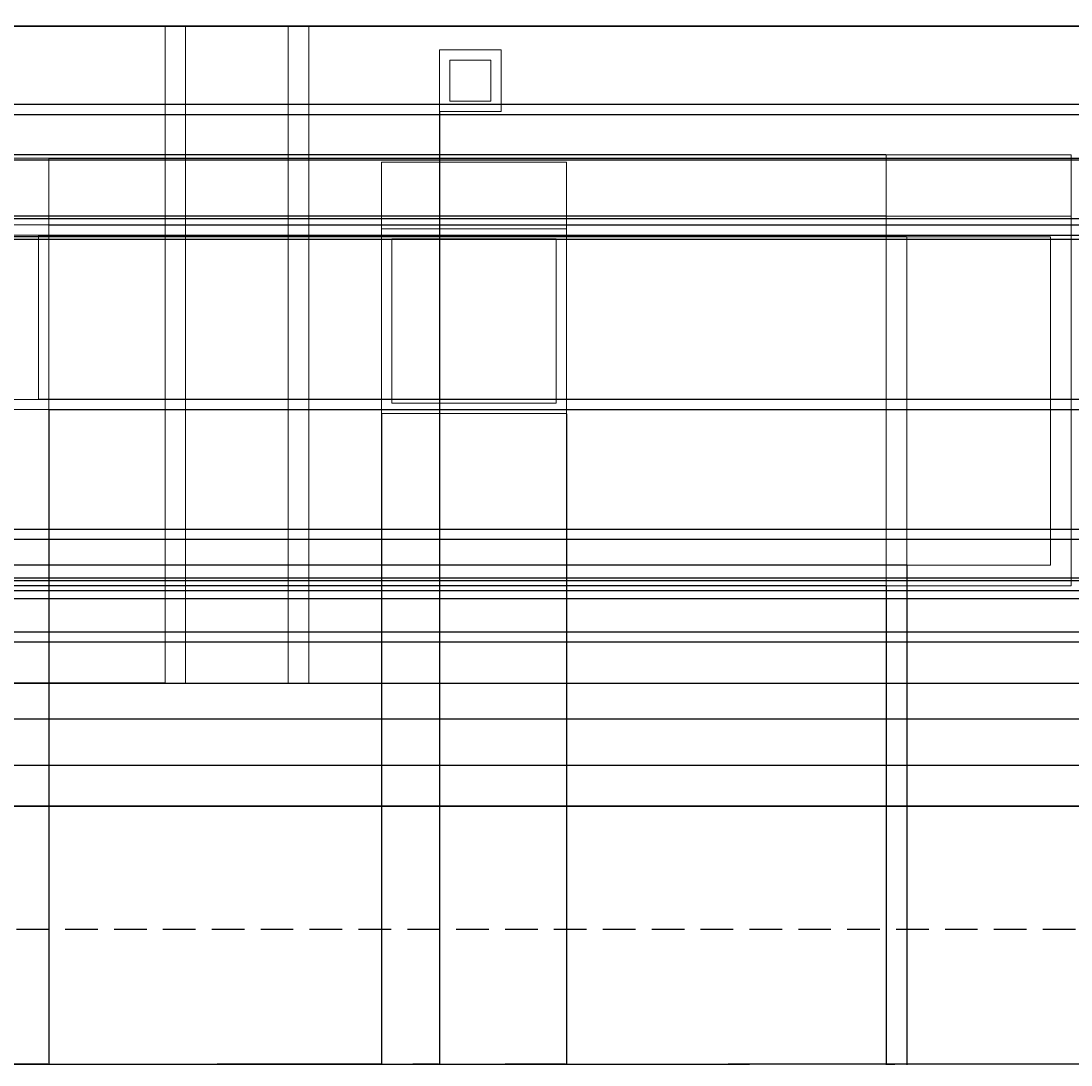
# Model space of a CAD drawing. Units: inches. Extents: x 1817 to 2378, y 1915 to 2370.
# Tile 3 of 8: x 1955 to 2160, y 1915 to 2119. Entities that reach past the tile are written whole.
import ezdxf

# ---------------------------------------------------------------- set-up
doc = ezdxf.new("R2010")
doc.units = ezdxf.units.IN
doc.linetypes.add('DASHED', pattern=[19.05, 12.7, -6.35])
doc.linetypes.add('DASHED2', pattern=[9.525, 6.35, -3.175])
for name, color, linetype, lineweight in [('A-ANNO-DIMS', 2, 'Continuous', 18), ('A-ELEV', 7, 'Continuous', 35), ('A-ELEV-HIDN', 8, 'DASHED', 18), ('A-GLAZ', 4, 'Continuous', 18), ('C-TOPO', 8, 'DASHED2', 25), ('P-PIPE', 6, 'Continuous', 18)]:
    doc.layers.add(name, color=color, linetype=linetype, lineweight=lineweight)
doc.styles.get("Standard").update_dxf_attribs({"font": 'arial.ttf'})
doc.dimstyles.get("Standard").update_dxf_attribs({"dimtxt": 0.18, "dimasz": 0.18, "dimexe": 0.18, "dimexo": 0.0625, "dimgap": 0.09, "dimtad": 0, "dimtih": 1, "dimtoh": 1, "dimdec": 4, "dimzin": 0, "dimdsep": 46, "dimtxsty": 'Standard', "dimcen": 0.09, "dimadec": 0, "dimazin": 0, "dimtfac": 1, "dimtdec": 4, "dimtofl": 0, "dimtmove": 0, "dimatfit": 3, "dimfxl": 1, "dimtolj": 1, "dimtzin": 0, "dimarcsym": 0})

# ---------------------------------------------------------------- blocks, each defined once
blk = doc.blocks.new('WIN-SQ-900')
for points in [[(1924.43, 2204.58), (1960.43, 2204.58), (1960.43, 2217.58), (1924.43, 2217.58)], [(1924.43, 2204.58), (1960.43, 2204.58), (1960.43, 2168.58), (1924.43, 2168.58)], [(1926.43, 2202.58), (1958.43, 2202.58), (1958.43, 2170.58), (1926.43, 2170.58)]]:
    blk.add_lwpolyline(points, close=True)
blk = doc.blocks.new('WIN-TALL-900')
for points in [[(2123.62, 2205.9), (2159.62, 2205.9), (2159.62, 2217.9), (2123.62, 2217.9)], [(2123.62, 2205.9), (2159.62, 2205.9), (2159.62, 2133.9), (2123.62, 2133.9)], [(2127.62, 2201.9), (2155.62, 2201.9), (2155.62, 2137.9), (2127.62, 2137.9)]]:
    blk.add_lwpolyline(points, close=True)
blk = doc.blocks.new('VENT-300')
for points in [[(1936.66, 2237.16), (1948.66, 2237.16), (1948.66, 2225.16), (1936.66, 2225.16)], [(1938.66, 2235.16), (1946.66, 2235.16), (1946.66, 2227.16), (1938.66, 2227.16)]]:
    blk.add_lwpolyline(points, close=True)
blk = doc.blocks.new('*D14')
at = {"layer": 'A-ANNO-DIMS', "color": 0, "lineweight": -2, "transparency": 16777216}
for p, q in [((1934.83, 2100.21), (1934.83, 1915.08)), ((1960.43, 2042.72), (1960.43, 1915.08)), ((1935.01, 1915.26), (1947.3, 1915.26)), ((1960.25, 1915.26), (1947.95, 1915.26))]:
    blk.add_line(p, q, dxfattribs=at)
at = {"layer": 'A-ANNO-DIMS', "color": 0, "transparency": 16777216}
for points in [[(1935.01, 1915.29), (1935.01, 1915.23), (1934.83, 1915.26)], [(1960.25, 1915.29), (1960.25, 1915.23), (1960.43, 1915.26)]]:
    blk.add_solid(points, dxfattribs=at)
at = {"layer": 'Defpoints', "color": 0, "transparency": 16777216}
for p in [(1934.83, 2100.28), (1960.43, 2042.79), (1960.43, 1915.26)]:
    blk.add_point(p, dxfattribs=at)
at = {"layer": 'A-ANNO-DIMS', "color": 0, "transparency": 16777216, "insert": (1947.63, 1915.26), "char_height": 0.18, "attachment_point": 5}
blk.add_mtext('\\A1;25.6', dxfattribs=at)
blk = doc.blocks.new('*D15')
at = {"layer": 'A-ANNO-DIMS', "color": 0, "lineweight": -2, "transparency": 16777216}
for p, q in [((1960.43, 2042.72), (1960.43, 1915.08)), ((2025.28, 2041.97), (2025.28, 1915.08)), ((1960.61, 1915.26), (1992.46, 1915.26)), ((2025.1, 1915.26), (1993.25, 1915.26))]:
    blk.add_line(p, q, dxfattribs=at)
at = {"layer": 'A-ANNO-DIMS', "color": 0, "transparency": 16777216}
for points in [[(1960.61, 1915.29), (1960.61, 1915.23), (1960.43, 1915.26)], [(2025.1, 1915.29), (2025.1, 1915.23), (2025.28, 1915.26)]]:
    blk.add_solid(points, dxfattribs=at)
at = {"layer": 'Defpoints', "color": 0, "transparency": 16777216}
for p in [(1960.43, 2042.79), (2025.28, 2042.03), (2025.28, 1915.26)]:
    blk.add_point(p, dxfattribs=at)
at = {"layer": 'A-ANNO-DIMS', "color": 0, "transparency": 16777216, "insert": (1992.85, 1915.26), "char_height": 0.18, "attachment_point": 5}
blk.add_mtext('\\A1;64.86', dxfattribs=at)
blk = doc.blocks.new('*D16')
at = {"layer": 'A-ANNO-DIMS', "color": 0, "lineweight": -2, "transparency": 16777216}
for p, q in [((2036.55, 2100.83), (2036.55, 1915.08)), ((2025.28, 2041.97), (2025.28, 1915.08)), ((2025.46, 1915.26), (2030.46, 1915.26)), ((2036.37, 1915.26), (2031.37, 1915.26))]:
    blk.add_line(p, q, dxfattribs=at)
at = {"layer": 'A-ANNO-DIMS', "color": 0, "transparency": 16777216}
for points in [[(2025.46, 1915.29), (2025.46, 1915.23), (2025.28, 1915.26)], [(2036.37, 1915.29), (2036.37, 1915.23), (2036.55, 1915.26)]]:
    blk.add_solid(points, dxfattribs=at)
at = {"layer": 'Defpoints', "color": 0, "transparency": 16777216}
for p in [(2036.55, 2100.89), (2025.28, 2042.03), (2036.55, 1915.26)]:
    blk.add_point(p, dxfattribs=at)
at = {"layer": 'A-ANNO-DIMS', "color": 0, "transparency": 16777216, "insert": (2030.91, 1915.26), "char_height": 0.18, "attachment_point": 5}
blk.add_mtext('\\A1;11.266', dxfattribs=at)
blk = doc.blocks.new('*D17')
at = {"layer": 'A-ANNO-DIMS', "color": 0, "lineweight": -2, "transparency": 16777216}
for p, q in [((2036.55, 2100.83), (2036.55, 1915.08)), ((2061.28, 2041.97), (2061.28, 1915.08)), ((2036.73, 1915.26), (2048.45, 1915.26)), ((2061.1, 1915.26), (2049.38, 1915.26))]:
    blk.add_line(p, q, dxfattribs=at)
at = {"layer": 'A-ANNO-DIMS', "color": 0, "transparency": 16777216}
for points in [[(2036.73, 1915.29), (2036.73, 1915.23), (2036.55, 1915.26)], [(2061.1, 1915.29), (2061.1, 1915.23), (2061.28, 1915.26)]]:
    blk.add_solid(points, dxfattribs=at)
at = {"layer": 'Defpoints', "color": 0, "transparency": 16777216}
for p in [(2036.55, 2100.89), (2061.28, 2042.03), (2061.28, 1915.26)]:
    blk.add_point(p, dxfattribs=at)
at = {"layer": 'A-ANNO-DIMS', "color": 0, "transparency": 16777216, "insert": (2048.91, 1915.26), "char_height": 0.18, "attachment_point": 5}
blk.add_mtext('\\A1;24.734', dxfattribs=at)
blk = doc.blocks.new('*D18')
at = {"layer": 'A-ANNO-DIMS', "color": 0, "lineweight": -2, "transparency": 16777216}
for p, q in [((2061.28, 2041.97), (2061.28, 1915.08)), ((2123.62, 2008.38), (2123.62, 1915.08)), ((2061.46, 1915.26), (2092.06, 1915.26)), ((2123.44, 1915.26), (2092.84, 1915.26))]:
    blk.add_line(p, q, dxfattribs=at)
at = {"layer": 'A-ANNO-DIMS', "color": 0, "transparency": 16777216}
for points in [[(2061.46, 1915.29), (2061.46, 1915.23), (2061.28, 1915.26)], [(2123.44, 1915.29), (2123.44, 1915.23), (2123.62, 1915.26)]]:
    blk.add_solid(points, dxfattribs=at)
at = {"layer": 'Defpoints', "color": 0, "transparency": 16777216}
for p in [(2061.28, 2042.03), (2123.62, 2008.45), (2123.62, 1915.26)]:
    blk.add_point(p, dxfattribs=at)
at = {"layer": 'A-ANNO-DIMS', "color": 0, "transparency": 16777216, "insert": (2092.45, 1915.26), "char_height": 0.18, "attachment_point": 5}
blk.add_mtext('\\A1;62.34', dxfattribs=at)
blk = doc.blocks.new('*D23')
at = {"layer": 'A-ANNO-DIMS', "color": 0, "lineweight": -2, "transparency": 16777216}
for p, q in [((2320.11, 2156.45), (2320.11, 1915.08)), ((1867.08, 1965.45), (1867.08, 1915.08)), ((1867.26, 1915.26), (2093.3, 1915.26)), ((2319.93, 1915.26), (2093.89, 1915.26))]:
    blk.add_line(p, q, dxfattribs=at)
at = {"layer": 'A-ANNO-DIMS', "color": 0, "transparency": 16777216}
for points in [[(1867.26, 1915.29), (1867.26, 1915.23), (1867.08, 1915.26)], [(2319.93, 1915.29), (2319.93, 1915.23), (2320.11, 1915.26)]]:
    blk.add_solid(points, dxfattribs=at)
at = {"layer": 'Defpoints', "color": 0, "transparency": 16777216}
for p in [(2320.11, 2156.51), (1867.08, 1965.51), (2320.11, 1915.26)]:
    blk.add_point(p, dxfattribs=at)
at = {"layer": 'A-ANNO-DIMS', "color": 0, "transparency": 16777216, "insert": (2093.6, 1915.26), "char_height": 0.18, "attachment_point": 5}
blk.add_mtext('\\A1;453', dxfattribs=at)
blk = doc.blocks.new('*D80')
at = {"layer": 'A-ANNO-DIMS', "color": 0, "lineweight": -2, "transparency": 16777216}
for p, q in [((2123.56, 2008.45), (1817.4, 2008.45)), ((1817.58, 2008.27), (1817.58, 1987.16)), ((1817.58, 1965.69), (1817.58, 1986.8)), ((2281.02, 1965.51), (1817.4, 1965.51))]:
    blk.add_line(p, q, dxfattribs=at)
at = {"layer": 'A-ANNO-DIMS', "color": 0, "transparency": 16777216}
for points in [[(1817.55, 2008.27), (1817.61, 2008.27), (1817.58, 2008.45)], [(1817.55, 1965.69), (1817.61, 1965.69), (1817.58, 1965.51)]]:
    blk.add_solid(points, dxfattribs=at)
at = {"layer": 'Defpoints', "color": 0, "transparency": 16777216}
for p in [(1817.58, 2008.45), (2123.62, 2008.45), (2281.08, 1965.51)]:
    blk.add_point(p, dxfattribs=at)
at = {"layer": 'A-ANNO-DIMS', "color": 0, "transparency": 16777216, "insert": (1817.58, 1986.98), "char_height": 0.18, "attachment_point": 5}
blk.add_mtext('\\A1;42.94', dxfattribs=at)
blk = doc.blocks.new('*D81')
at = {"layer": 'A-ANNO-DIMS', "color": 0, "lineweight": -2, "transparency": 16777216}
for p, q in [((2198.53, 2117.51), (1817.4, 2117.51)), ((1817.58, 2117.33), (1817.58, 2105.16)), ((1817.58, 2092.63), (1817.58, 2104.8)), ((2123.56, 2092.45), (1817.4, 2092.45))]:
    blk.add_line(p, q, dxfattribs=at)
at = {"layer": 'A-ANNO-DIMS', "color": 0, "transparency": 16777216}
for points in [[(1817.55, 2117.33), (1817.61, 2117.33), (1817.58, 2117.51)], [(1817.55, 2092.63), (1817.61, 2092.63), (1817.58, 2092.45)]]:
    blk.add_solid(points, dxfattribs=at)
at = {"layer": 'Defpoints', "color": 0, "transparency": 16777216}
for p in [(1817.58, 2117.51), (2198.59, 2117.51), (2123.62, 2092.45)]:
    blk.add_point(p, dxfattribs=at)
at = {"layer": 'A-ANNO-DIMS', "color": 0, "transparency": 16777216, "insert": (1817.58, 2104.98), "char_height": 0.18, "attachment_point": 5}
blk.add_mtext('\\A1;25.06', dxfattribs=at)
blk = doc.blocks.new('*D84')
at = {"layer": 'A-ANNO-DIMS', "color": 0, "lineweight": -2, "transparency": 16777216}
for p, q in [((1960.49, 2091.79), (2377.4, 2091.79)), ((2377.22, 2091.61), (2377.22, 2085.47)), ((2377.22, 2078.97), (2377.22, 2085.1)), ((1960.49, 2078.79), (2377.4, 2078.79))]:
    blk.add_line(p, q, dxfattribs=at)
at = {"layer": 'A-ANNO-DIMS', "color": 0, "transparency": 16777216}
for points in [[(2377.19, 2091.61), (2377.25, 2091.61), (2377.22, 2091.79)], [(2377.19, 2078.97), (2377.25, 2078.97), (2377.22, 2078.79)]]:
    blk.add_solid(points, dxfattribs=at)
at = {"layer": 'Defpoints', "color": 0, "transparency": 16777216}
for p in [(1960.43, 2091.79), (1960.43, 2078.79), (2377.22, 2078.79)]:
    blk.add_point(p, dxfattribs=at)
at = {"layer": 'A-ANNO-DIMS', "color": 0, "transparency": 16777216, "insert": (2377.22, 2085.29), "char_height": 0.18, "attachment_point": 5}
blk.add_mtext('\\A1;13.00', dxfattribs=at)
blk = doc.blocks.new('*D85')
at = {"layer": 'A-ANNO-DIMS', "color": 0, "lineweight": -2, "transparency": 16777216}
for p, q in [((1960.49, 2078.79), (2377.4, 2078.79)), ((2377.22, 2078.61), (2377.22, 2077.97)), ((2377.22, 2076.97), (2377.22, 2077.6)), ((1958.49, 2076.79), (2377.4, 2076.79))]:
    blk.add_line(p, q, dxfattribs=at)
at = {"layer": 'A-ANNO-DIMS', "color": 0, "transparency": 16777216}
for points in [[(2377.19, 2078.61), (2377.25, 2078.61), (2377.22, 2078.79)], [(2377.19, 2076.97), (2377.25, 2076.97), (2377.22, 2076.79)]]:
    blk.add_solid(points, dxfattribs=at)
at = {"layer": 'Defpoints', "color": 0, "transparency": 16777216}
for p in [(1960.43, 2078.79), (1958.43, 2076.79), (2377.22, 2076.79)]:
    blk.add_point(p, dxfattribs=at)
at = {"layer": 'A-ANNO-DIMS', "color": 0, "transparency": 16777216, "insert": (2377.22, 2077.79), "char_height": 0.18, "attachment_point": 5}
blk.add_mtext('\\A1;2.00', dxfattribs=at)
blk = doc.blocks.new('*D86')
at = {"layer": 'A-ANNO-DIMS', "color": 0, "lineweight": -2, "transparency": 16777216}
for p, q in [((1958.49, 2044.79), (2377.4, 2044.79)), ((2377.22, 2044.61), (2377.22, 2043.97)), ((1960.49, 2042.79), (2377.4, 2042.79)), ((2377.22, 2042.97), (2377.22, 2043.6))]:
    blk.add_line(p, q, dxfattribs=at)
at = {"layer": 'A-ANNO-DIMS', "color": 0, "transparency": 16777216}
for points in [[(2377.19, 2044.61), (2377.25, 2044.61), (2377.22, 2044.79)], [(2377.19, 2042.97), (2377.25, 2042.97), (2377.22, 2042.79)]]:
    blk.add_solid(points, dxfattribs=at)
at = {"layer": 'Defpoints', "color": 0, "transparency": 16777216}
for p in [(1958.43, 2044.79), (1960.43, 2042.79), (2377.22, 2042.79)]:
    blk.add_point(p, dxfattribs=at)
at = {"layer": 'A-ANNO-DIMS', "color": 0, "transparency": 16777216, "insert": (2377.22, 2043.79), "char_height": 0.18, "attachment_point": 5}
blk.add_mtext('\\A1;2.00', dxfattribs=at)
blk = doc.blocks.new('*D89')
at = {"layer": 'A-ANNO-DIMS', "color": 0, "lineweight": -2, "transparency": 16777216}
for p, q in [((1944.89, 2102.28), (2377.4, 2102.28)), ((2377.22, 2102.1), (2377.22, 2101.46)), ((1946.89, 2100.28), (2377.4, 2100.28)), ((2377.22, 2100.46), (2377.22, 2101.09))]:
    blk.add_line(p, q, dxfattribs=at)
at = {"layer": 'A-ANNO-DIMS', "color": 0, "transparency": 16777216}
for points in [[(2377.19, 2102.1), (2377.25, 2102.1), (2377.22, 2102.28)], [(2377.19, 2100.46), (2377.25, 2100.46), (2377.22, 2100.28)]]:
    blk.add_solid(points, dxfattribs=at)
at = {"layer": 'Defpoints', "color": 0, "transparency": 16777216}
for p in [(1944.83, 2102.28), (2377.22, 2102.28), (1946.83, 2100.28)]:
    blk.add_point(p, dxfattribs=at)
at = {"layer": 'A-ANNO-DIMS', "color": 0, "transparency": 16777216, "insert": (2377.22, 2101.28), "char_height": 0.18, "attachment_point": 5}
blk.add_mtext('\\A1;2.00', dxfattribs=at)
blk = doc.blocks.new('*D90')
at = {"layer": 'A-ANNO-DIMS', "color": 0, "lineweight": -2, "transparency": 16777216}
for p, q in [((2123.56, 2092.45), (1817.4, 2092.45)), ((1817.58, 2092.27), (1817.58, 2086.63)), ((1817.58, 2080.63), (1817.58, 2086.26)), ((2123.56, 2080.45), (1817.4, 2080.45))]:
    blk.add_line(p, q, dxfattribs=at)
at = {"layer": 'A-ANNO-DIMS', "color": 0, "transparency": 16777216}
for points in [[(1817.55, 2092.27), (1817.61, 2092.27), (1817.58, 2092.45)], [(1817.55, 2080.63), (1817.61, 2080.63), (1817.58, 2080.45)]]:
    blk.add_solid(points, dxfattribs=at)
at = {"layer": 'Defpoints', "color": 0, "transparency": 16777216}
for p in [(2123.62, 2092.45), (1817.58, 2080.45), (2123.62, 2080.45)]:
    blk.add_point(p, dxfattribs=at)
at = {"layer": 'A-ANNO-DIMS', "color": 0, "transparency": 16777216, "insert": (1817.58, 2086.45), "char_height": 0.18, "attachment_point": 5}
blk.add_mtext('\\A1;12.00', dxfattribs=at)
blk = doc.blocks.new('*D91')
at = {"layer": 'A-ANNO-DIMS', "color": 0, "lineweight": -2, "transparency": 16777216}
for p, q in [((2123.56, 2080.45), (1817.4, 2080.45)), ((1817.58, 2080.27), (1817.58, 2078.63)), ((1817.58, 2076.63), (1817.58, 2078.26)), ((2127.56, 2076.45), (1817.4, 2076.45))]:
    blk.add_line(p, q, dxfattribs=at)
at = {"layer": 'A-ANNO-DIMS', "color": 0, "transparency": 16777216}
for points in [[(1817.55, 2080.27), (1817.61, 2080.27), (1817.58, 2080.45)], [(1817.55, 2076.63), (1817.61, 2076.63), (1817.58, 2076.45)]]:
    blk.add_solid(points, dxfattribs=at)
at = {"layer": 'Defpoints', "color": 0, "transparency": 16777216}
for p in [(2123.62, 2080.45), (1817.58, 2076.45), (2127.62, 2076.45)]:
    blk.add_point(p, dxfattribs=at)
at = {"layer": 'A-ANNO-DIMS', "color": 0, "transparency": 16777216, "insert": (1817.58, 2078.45), "char_height": 0.18, "attachment_point": 5}
blk.add_mtext('\\A1;4.00', dxfattribs=at)
blk = doc.blocks.new('*D92')
at = {"layer": 'A-ANNO-DIMS', "color": 0, "lineweight": -2, "transparency": 16777216}
for p, q in [((2127.56, 2012.45), (1817.4, 2012.45)), ((1817.58, 2012.27), (1817.58, 2010.63)), ((1817.58, 2008.63), (1817.58, 2010.26)), ((2123.56, 2008.45), (1817.4, 2008.45))]:
    blk.add_line(p, q, dxfattribs=at)
at = {"layer": 'A-ANNO-DIMS', "color": 0, "transparency": 16777216}
for points in [[(1817.55, 2012.27), (1817.61, 2012.27), (1817.58, 2012.45)], [(1817.55, 2008.63), (1817.61, 2008.63), (1817.58, 2008.45)]]:
    blk.add_solid(points, dxfattribs=at)
at = {"layer": 'Defpoints', "color": 0, "transparency": 16777216}
for p in [(2127.62, 2012.45), (1817.58, 2008.45), (2123.62, 2008.45)]:
    blk.add_point(p, dxfattribs=at)
at = {"layer": 'A-ANNO-DIMS', "color": 0, "transparency": 16777216, "insert": (1817.58, 2010.45), "char_height": 0.18, "attachment_point": 5}
blk.add_mtext('\\A1;4.00', dxfattribs=at)
blk = doc.blocks.new('*D93')
at = {"layer": 'A-ANNO-DIMS', "color": 0, "lineweight": -2, "transparency": 16777216}
for p, q in [((2127.62, 2012.38), (2127.62, 1915.08)), ((2123.62, 2008.38), (2123.62, 1915.08)), ((2123.8, 1915.26), (2125.29, 1915.26)), ((2127.44, 1915.26), (2125.94, 1915.26))]:
    blk.add_line(p, q, dxfattribs=at)
at = {"layer": 'A-ANNO-DIMS', "color": 0, "transparency": 16777216}
for points in [[(2123.8, 1915.29), (2123.8, 1915.23), (2123.62, 1915.26)], [(2127.44, 1915.29), (2127.44, 1915.23), (2127.62, 1915.26)]]:
    blk.add_solid(points, dxfattribs=at)
at = {"layer": 'Defpoints', "color": 0, "transparency": 16777216}
for p in [(2127.62, 2012.45), (2123.62, 2008.45), (2127.62, 1915.26)]:
    blk.add_point(p, dxfattribs=at)
at = {"layer": 'A-ANNO-DIMS', "color": 0, "transparency": 16777216, "insert": (2125.62, 1915.26), "char_height": 0.18, "attachment_point": 5}
blk.add_mtext('\\A1;4.00', dxfattribs=at)
blk = doc.blocks.new('*D94')
at = {"layer": 'A-ANNO-DIMS', "color": 0, "lineweight": -2, "transparency": 16777216}
for p, q in [((2210.55, 2091.36), (1817.4, 2091.36)), ((1817.58, 2091.18), (1817.58, 2085.83)), ((1817.58, 2080.11), (1817.58, 2085.47)), ((2210.55, 2079.93), (1817.4, 2079.93))]:
    blk.add_line(p, q, dxfattribs=at)
at = {"layer": 'A-ANNO-DIMS', "color": 0, "transparency": 16777216}
for points in [[(1817.55, 2091.18), (1817.61, 2091.18), (1817.58, 2091.36)], [(1817.55, 2080.11), (1817.61, 2080.11), (1817.58, 2079.93)]]:
    blk.add_solid(points, dxfattribs=at)
at = {"layer": 'Defpoints', "color": 0, "transparency": 16777216}
for p in [(2210.62, 2091.36), (1817.58, 2079.93), (2210.62, 2079.93)]:
    blk.add_point(p, dxfattribs=at)
at = {"layer": 'A-ANNO-DIMS', "color": 0, "transparency": 16777216, "insert": (1817.58, 2085.65), "char_height": 0.18, "attachment_point": 5}
blk.add_mtext('\\A1;11.433', dxfattribs=at)
blk = doc.blocks.new('*D95')
at = {"layer": 'A-ANNO-DIMS', "color": 0, "lineweight": -2, "transparency": 16777216}
for p, q in [((2210.55, 2079.93), (1817.4, 2079.93)), ((1817.58, 2079.75), (1817.58, 2078.11)), ((1817.58, 2076.11), (1817.58, 2077.75)), ((2214.55, 2075.93), (1817.4, 2075.93))]:
    blk.add_line(p, q, dxfattribs=at)
at = {"layer": 'A-ANNO-DIMS', "color": 0, "transparency": 16777216}
for points in [[(1817.55, 2079.75), (1817.61, 2079.75), (1817.58, 2079.93)], [(1817.55, 2076.11), (1817.61, 2076.11), (1817.58, 2075.93)]]:
    blk.add_solid(points, dxfattribs=at)
at = {"layer": 'Defpoints', "color": 0, "transparency": 16777216}
for p in [(2210.62, 2079.93), (1817.58, 2075.93), (2214.62, 2075.93)]:
    blk.add_point(p, dxfattribs=at)
at = {"layer": 'A-ANNO-DIMS', "color": 0, "transparency": 16777216, "insert": (1817.58, 2077.93), "char_height": 0.18, "attachment_point": 5}
blk.add_mtext('\\A1;4.00', dxfattribs=at)
blk = doc.blocks.new('*D96')
at = {"layer": 'A-ANNO-DIMS', "color": 0, "lineweight": -2, "transparency": 16777216}
for p, q in [((2214.55, 2009.93), (1817.4, 2009.93)), ((1817.58, 2009.75), (1817.58, 2008.11)), ((1817.58, 2006.11), (1817.58, 2007.75)), ((2210.55, 2005.93), (1817.4, 2005.93))]:
    blk.add_line(p, q, dxfattribs=at)
at = {"layer": 'A-ANNO-DIMS', "color": 0, "transparency": 16777216}
for points in [[(1817.55, 2009.75), (1817.61, 2009.75), (1817.58, 2009.93)], [(1817.55, 2006.11), (1817.61, 2006.11), (1817.58, 2005.93)]]:
    blk.add_solid(points, dxfattribs=at)
at = {"layer": 'Defpoints', "color": 0, "transparency": 16777216}
for p in [(2214.62, 2009.93), (1817.58, 2005.93), (2210.62, 2005.93)]:
    blk.add_point(p, dxfattribs=at)
at = {"layer": 'A-ANNO-DIMS', "color": 0, "transparency": 16777216, "insert": (1817.58, 2007.93), "char_height": 0.18, "attachment_point": 5}
blk.add_mtext('\\A1;4.00', dxfattribs=at)
blk = doc.blocks.new('*D107')
at = {"layer": 'A-ANNO-DIMS', "color": 0, "lineweight": -2, "transparency": 16777216}
for p, q in [((1903.15, 2019.51), (2377.4, 2019.51)), ((2377.22, 2019.33), (2377.22, 2018.69)), ((2377.22, 2017.69), (2377.22, 2018.33)), ((1903.15, 2017.51), (2377.4, 2017.51))]:
    blk.add_line(p, q, dxfattribs=at)
at = {"layer": 'A-ANNO-DIMS', "color": 0, "transparency": 16777216}
for points in [[(2377.19, 2019.33), (2377.25, 2019.33), (2377.22, 2019.51)], [(2377.19, 2017.69), (2377.25, 2017.69), (2377.22, 2017.51)]]:
    blk.add_solid(points, dxfattribs=at)
at = {"layer": 'Defpoints', "color": 0, "transparency": 16777216}
for p in [(1903.08, 2019.51), (1903.08, 2017.51), (2377.22, 2017.51)]:
    blk.add_point(p, dxfattribs=at)
at = {"layer": 'A-ANNO-DIMS', "color": 0, "transparency": 16777216, "insert": (2377.22, 2018.51), "char_height": 0.18, "attachment_point": 5}
blk.add_mtext('\\A1;2.00', dxfattribs=at)
blk = doc.blocks.new('*D108')
at = {"layer": 'A-ANNO-DIMS', "color": 0, "lineweight": -2, "transparency": 16777216}
for p, q in [((1903.15, 2017.51), (2377.4, 2017.51)), ((2377.22, 2017.33), (2377.22, 2013.69)), ((2377.22, 2009.69), (2377.22, 2013.33)), ((1903.15, 2009.51), (2377.4, 2009.51))]:
    blk.add_line(p, q, dxfattribs=at)
at = {"layer": 'A-ANNO-DIMS', "color": 0, "transparency": 16777216}
for points in [[(2377.19, 2017.33), (2377.25, 2017.33), (2377.22, 2017.51)], [(2377.19, 2009.69), (2377.25, 2009.69), (2377.22, 2009.51)]]:
    blk.add_solid(points, dxfattribs=at)
at = {"layer": 'Defpoints', "color": 0, "transparency": 16777216}
for p in [(1903.08, 2017.51), (1903.08, 2009.51), (2377.22, 2009.51)]:
    blk.add_point(p, dxfattribs=at)
at = {"layer": 'A-ANNO-DIMS', "color": 0, "transparency": 16777216, "insert": (2377.22, 2013.51), "char_height": 0.18, "attachment_point": 5}
blk.add_mtext('\\A1;8.00', dxfattribs=at)
blk = doc.blocks.new('*D109')
at = {"layer": 'A-ANNO-DIMS', "color": 0, "lineweight": -2, "transparency": 16777216}
for p, q in [((1903.15, 2009.51), (2377.4, 2009.51)), ((1903.15, 2007.51), (2377.4, 2007.51)), ((2377.22, 2009.33), (2377.22, 2008.69)), ((2377.22, 2007.69), (2377.22, 2008.33))]:
    blk.add_line(p, q, dxfattribs=at)
at = {"layer": 'A-ANNO-DIMS', "color": 0, "transparency": 16777216}
for points in [[(2377.19, 2009.33), (2377.25, 2009.33), (2377.22, 2009.51)], [(2377.19, 2007.69), (2377.25, 2007.69), (2377.22, 2007.51)]]:
    blk.add_solid(points, dxfattribs=at)
at = {"layer": 'Defpoints', "color": 0, "transparency": 16777216}
for p in [(1903.08, 2009.51), (1903.08, 2007.51), (2377.22, 2007.51)]:
    blk.add_point(p, dxfattribs=at)
at = {"layer": 'A-ANNO-DIMS', "color": 0, "transparency": 16777216, "insert": (2377.22, 2008.51), "char_height": 0.18, "attachment_point": 5}
blk.add_mtext('\\A1;2.00', dxfattribs=at)
blk = doc.blocks.new('*D110')
at = {"layer": 'A-ANNO-DIMS', "color": 0, "lineweight": -2, "transparency": 16777216}
for p, q in [((1903.15, 2007.51), (2377.4, 2007.51)), ((2377.22, 2007.33), (2377.22, 2003.69)), ((2377.22, 1999.69), (2377.22, 2003.33)), ((1903.15, 1999.51), (2377.4, 1999.51))]:
    blk.add_line(p, q, dxfattribs=at)
at = {"layer": 'A-ANNO-DIMS', "color": 0, "transparency": 16777216}
for points in [[(2377.19, 2007.33), (2377.25, 2007.33), (2377.22, 2007.51)], [(2377.19, 1999.69), (2377.25, 1999.69), (2377.22, 1999.51)]]:
    blk.add_solid(points, dxfattribs=at)
at = {"layer": 'Defpoints', "color": 0, "transparency": 16777216}
for p in [(1903.08, 2007.51), (1903.08, 1999.51), (2377.22, 1999.51)]:
    blk.add_point(p, dxfattribs=at)
at = {"layer": 'A-ANNO-DIMS', "color": 0, "transparency": 16777216, "insert": (2377.22, 2003.51), "char_height": 0.18, "attachment_point": 5}
blk.add_mtext('\\A1;8.00', dxfattribs=at)
blk = doc.blocks.new('*D111')
at = {"layer": 'A-ANNO-DIMS', "color": 0, "lineweight": -2, "transparency": 16777216}
for p, q in [((1903.15, 1999.51), (2377.4, 1999.51)), ((2377.22, 1999.33), (2377.22, 1998.69)), ((1903.15, 1997.51), (2377.4, 1997.51)), ((2377.22, 1997.69), (2377.22, 1998.33))]:
    blk.add_line(p, q, dxfattribs=at)
at = {"layer": 'A-ANNO-DIMS', "color": 0, "transparency": 16777216}
for points in [[(2377.19, 1999.33), (2377.25, 1999.33), (2377.22, 1999.51)], [(2377.19, 1997.69), (2377.25, 1997.69), (2377.22, 1997.51)]]:
    blk.add_solid(points, dxfattribs=at)
at = {"layer": 'Defpoints', "color": 0, "transparency": 16777216}
for p in [(1903.08, 1999.51), (1903.08, 1997.51), (2377.22, 1997.51)]:
    blk.add_point(p, dxfattribs=at)
at = {"layer": 'A-ANNO-DIMS', "color": 0, "transparency": 16777216, "insert": (2377.22, 1998.51), "char_height": 0.18, "attachment_point": 5}
blk.add_mtext('\\A1;2.00', dxfattribs=at)
blk = doc.blocks.new('*D112')
at = {"layer": 'A-ANNO-DIMS', "color": 0, "lineweight": -2, "transparency": 16777216}
for p, q in [((1903.15, 1997.51), (2377.4, 1997.51)), ((2377.22, 1997.33), (2377.22, 1993.69)), ((2377.22, 1989.69), (2377.22, 1993.33)), ((1903.15, 1989.51), (2377.4, 1989.51))]:
    blk.add_line(p, q, dxfattribs=at)
at = {"layer": 'A-ANNO-DIMS', "color": 0, "transparency": 16777216}
for points in [[(2377.19, 1997.33), (2377.25, 1997.33), (2377.22, 1997.51)], [(2377.19, 1989.69), (2377.25, 1989.69), (2377.22, 1989.51)]]:
    blk.add_solid(points, dxfattribs=at)
at = {"layer": 'Defpoints', "color": 0, "transparency": 16777216}
for p in [(1903.08, 1997.51), (1903.08, 1989.51), (2377.22, 1989.51)]:
    blk.add_point(p, dxfattribs=at)
at = {"layer": 'A-ANNO-DIMS', "color": 0, "transparency": 16777216, "insert": (2377.22, 1993.51), "char_height": 0.18, "attachment_point": 5}
blk.add_mtext('\\A1;8.00', dxfattribs=at)
blk = doc.blocks.new('*D113')
at = {"layer": 'A-ANNO-DIMS', "color": 0, "lineweight": -2, "transparency": 16777216}
for p, q in [((1903.15, 1989.51), (2377.4, 1989.51)), ((2377.22, 1989.33), (2377.22, 1986.19)), ((2377.22, 1982.69), (2377.22, 1985.83)), ((1903.15, 1982.51), (2377.4, 1982.51))]:
    blk.add_line(p, q, dxfattribs=at)
at = {"layer": 'A-ANNO-DIMS', "color": 0, "transparency": 16777216}
for points in [[(2377.19, 1989.33), (2377.25, 1989.33), (2377.22, 1989.51)], [(2377.19, 1982.69), (2377.25, 1982.69), (2377.22, 1982.51)]]:
    blk.add_solid(points, dxfattribs=at)
at = {"layer": 'Defpoints', "color": 0, "transparency": 16777216}
for p in [(1903.08, 1989.51), (1903.08, 1982.51), (2377.22, 1982.51)]:
    blk.add_point(p, dxfattribs=at)
at = {"layer": 'A-ANNO-DIMS', "color": 0, "transparency": 16777216, "insert": (2377.22, 1986.01), "char_height": 0.18, "attachment_point": 5}
blk.add_mtext('\\A1;7.00', dxfattribs=at)
blk = doc.blocks.new('*D114')
at = {"layer": 'A-ANNO-DIMS', "color": 0, "lineweight": -2, "transparency": 16777216}
for p, q in [((1903.15, 1982.51), (2377.4, 1982.51)), ((2377.22, 1982.33), (2377.22, 1978.19)), ((2377.22, 1973.69), (2377.22, 1977.83)), ((1903.15, 1973.51), (2377.4, 1973.51))]:
    blk.add_line(p, q, dxfattribs=at)
at = {"layer": 'A-ANNO-DIMS', "color": 0, "transparency": 16777216}
for points in [[(2377.19, 1982.33), (2377.25, 1982.33), (2377.22, 1982.51)], [(2377.19, 1973.69), (2377.25, 1973.69), (2377.22, 1973.51)]]:
    blk.add_solid(points, dxfattribs=at)
at = {"layer": 'Defpoints', "color": 0, "transparency": 16777216}
for p in [(1903.08, 1982.51), (1903.08, 1973.51), (2377.22, 1973.51)]:
    blk.add_point(p, dxfattribs=at)
at = {"layer": 'A-ANNO-DIMS', "color": 0, "transparency": 16777216, "insert": (2377.22, 1978.01), "char_height": 0.18, "attachment_point": 5}
blk.add_mtext('\\A1;9.00', dxfattribs=at)
blk = doc.blocks.new('*D115')
at = {"layer": 'A-ANNO-DIMS', "color": 0, "lineweight": -2, "transparency": 16777216}
for p, q in [((1903.15, 1973.51), (2377.4, 1973.51)), ((2377.22, 1973.33), (2377.22, 1969.69)), ((2377.22, 1965.69), (2377.22, 1969.33)), ((1903.15, 1965.51), (2377.4, 1965.51))]:
    blk.add_line(p, q, dxfattribs=at)
at = {"layer": 'A-ANNO-DIMS', "color": 0, "transparency": 16777216}
for points in [[(2377.19, 1973.33), (2377.25, 1973.33), (2377.22, 1973.51)], [(2377.19, 1965.69), (2377.25, 1965.69), (2377.22, 1965.51)]]:
    blk.add_solid(points, dxfattribs=at)
at = {"layer": 'Defpoints', "color": 0, "transparency": 16777216}
for p in [(1903.08, 1973.51), (1903.08, 1965.51), (2377.22, 1965.51)]:
    blk.add_point(p, dxfattribs=at)
at = {"layer": 'A-ANNO-DIMS', "color": 0, "transparency": 16777216, "insert": (2377.22, 1969.51), "char_height": 0.18, "attachment_point": 5}
blk.add_mtext('\\A1;8.00', dxfattribs=at)
blk = doc.blocks.new('*D118')
at = {"layer": 'A-ANNO-DIMS', "color": 0, "lineweight": -2, "transparency": 16777216}
for p, q in [((1843.83, 1941.45), (1843.83, 1915.08)), ((2350.97, 1941.45), (2350.97, 1915.08)), ((1844.01, 1915.26), (2096.94, 1915.26)), ((2350.79, 1915.26), (2097.86, 1915.26))]:
    blk.add_line(p, q, dxfattribs=at)
at = {"layer": 'A-ANNO-DIMS', "color": 0, "transparency": 16777216}
for points in [[(1844.01, 1915.29), (1844.01, 1915.23), (1843.83, 1915.26)], [(2350.79, 1915.29), (2350.79, 1915.23), (2350.97, 1915.26)]]:
    blk.add_solid(points, dxfattribs=at)
at = {"layer": 'Defpoints', "color": 0, "transparency": 16777216}
for p in [(1843.83, 1941.51), (2350.97, 1941.51), (2350.97, 1915.26)]:
    blk.add_point(p, dxfattribs=at)
at = {"layer": 'A-ANNO-DIMS', "color": 0, "transparency": 16777216, "insert": (2097.4, 1915.26), "char_height": 0.18, "attachment_point": 5}
blk.add_mtext('\\A1;507.13', dxfattribs=at)
blk = doc.blocks.new('*D119')
at = {"layer": 'A-ANNO-DIMS', "color": 0, "lineweight": -2, "transparency": 16777216}
for p, q in [((1903.08, 1989.57), (1903.08, 2369.94)), ((1903.26, 2369.76), (2091.62, 2369.76)), ((2280.9, 2369.76), (2092.55, 2369.76)), ((2281.08, 1989.57), (2281.08, 2369.94))]:
    blk.add_line(p, q, dxfattribs=at)
at = {"layer": 'A-ANNO-DIMS', "color": 0, "transparency": 16777216}
for points in [[(1903.26, 2369.79), (1903.26, 2369.73), (1903.08, 2369.76)], [(2280.9, 2369.79), (2280.9, 2369.73), (2281.08, 2369.76)]]:
    blk.add_solid(points, dxfattribs=at)
at = {"layer": 'Defpoints', "color": 0, "transparency": 16777216}
for p in [(2281.08, 2369.76), (1903.08, 1989.51), (2281.08, 1989.51)]:
    blk.add_point(p, dxfattribs=at)
at = {"layer": 'A-ANNO-DIMS', "color": 0, "transparency": 16777216, "insert": (2092.08, 2369.76), "char_height": 0.18, "attachment_point": 5}
blk.add_mtext('\\A1;378.00', dxfattribs=at)
blk = doc.blocks.new('*D120')
at = {"layer": 'A-ANNO-DIMS', "color": 0, "lineweight": -2, "transparency": 16777216}
for p, q in [((1983.02, 2117.51), (1817.4, 2117.51)), ((1817.58, 2117.33), (1817.58, 2053.69)), ((1817.58, 1989.69), (1817.58, 2053.33)), ((1983.02, 1989.51), (1817.4, 1989.51))]:
    blk.add_line(p, q, dxfattribs=at)
at = {"layer": 'A-ANNO-DIMS', "color": 0, "transparency": 16777216}
for points in [[(1817.55, 2117.33), (1817.61, 2117.33), (1817.58, 2117.51)], [(1817.55, 1989.69), (1817.61, 1989.69), (1817.58, 1989.51)]]:
    blk.add_solid(points, dxfattribs=at)
at = {"layer": 'Defpoints', "color": 0, "transparency": 16777216}
for p in [(1817.58, 2117.51), (1983.08, 2117.51), (1983.08, 1989.51)]:
    blk.add_point(p, dxfattribs=at)
at = {"layer": 'A-ANNO-DIMS', "color": 0, "transparency": 16777216, "insert": (1817.58, 2053.51), "char_height": 0.18, "attachment_point": 5}
blk.add_mtext('\\A1;128.00', dxfattribs=at)

msp = doc.modelspace()

# ---------------------------------------------------------------- linework, layer by layer
at = {"layer": 'A-ELEV'}
msp.add_line((2198.5896, 2117.5087), (1895.6961, 2117.5087), dxfattribs=at)
at = {"layer": 'A-ELEV-HIDN'}
msp.add_line((2281.0849, 1989.5087), (1903.0849, 1989.5087), dxfattribs=at)
at = {"layer": 'C-TOPO'}
for p, q in [((2281.0849, 1965.5087), (1867.0849, 1965.5087)), ((2350.9681, 1941.5087), (1843.834, 1941.5087))]:
    msp.add_line(p, q, dxfattribs=at)
at = {"layer": 'P-PIPE'}
for p, q in [((1983.0849, 1989.5087), (1983.0849, 2117.5087)), ((1987.0849, 1989.5087), (1987.0849, 2117.5087)), ((2007.0849, 1989.5087), (2007.0849, 2117.5087)), ((2011.0849, 1989.5087), (2011.0849, 2117.5087))]:
    msp.add_line(p, q, dxfattribs=at)

# ---------------------------------------------------------------- block references
at = {"layer": 'A-GLAZ'}
for name, p in [('VENT-300', (99.8818, -124.2714)), ('WIN-SQ-900', (0, -125.7955)), ('WIN-TALL-900', (0, -125.4487)), ('WIN-SQ-900', (100.8553, -126.5465))]:
    msp.add_blockref(name, p, dxfattribs=at)

# ---------------------------------------------------------------- dimensions: what is measured, and where the dimension line sits
at = {"layer": 'A-ANNO-DIMS'}
for base, p1, p2, override, picture, middle in [((2281.0849, 2369.7587), (1903.0849, 1989.5087), (2281.0849, 1989.5087), {"dimdec": 2, "dimlfac": 1, "dimrnd": 0, "dimzin": 0, "dimdsep": 46, "dimlunit": 2}, '*D119', (2092.0849, 2369.7587)), ((2320.1054, 1915.2587), (1867.0849, 1965.5087), (2320.1054, 2156.5133), {"dimdec": 0, "dimlfac": 1, "dimrnd": 0, "dimzin": 0, "dimdsep": 46, "dimlunit": 2}, '*D23', (2093.5951, 1915.2587)), ((1960.4258, 1915.2587), (1934.8265, 2100.2756), (1960.4258, 2042.7858), {"dimdec": 1, "dimlfac": 1, "dimrnd": 0, "dimzin": 0, "dimdsep": 46, "dimlunit": 2}, '*D14', (1947.6262, 1915.2587)), ((2036.54663, 1915.25873), (2025.28107, 2042.03485), (2036.54663, 2100.88778), {"dimdec": 3, "dimlfac": 1, "dimrnd": 0, "dimzin": 0, "dimdsep": 46, "dimlunit": 2}, '*D16', (2030.91385, 1915.25873)), ((2061.28107, 1915.25873), (2036.54663, 2100.88778), (2061.28107, 2042.03485), {"dimdec": 3, "dimlfac": 1, "dimrnd": 0, "dimzin": 0, "dimdsep": 46, "dimlunit": 2}, '*D17', (2048.91385, 1915.25873)), ((2025.2811, 1915.2587), (1960.4258, 2042.7858), (2025.2811, 2042.0349), {"dimdec": 2, "dimlfac": 1, "dimrnd": 0, "dimzin": 0, "dimdsep": 46, "dimlunit": 2}, '*D15', (1992.8534, 1915.2587)), ((2123.6179, 1915.2587), (2061.2811, 2042.0349), (2123.6179, 2008.4468), {"dimdec": 2, "dimlfac": 1, "dimrnd": 0, "dimzin": 0, "dimdsep": 46, "dimlunit": 2}, '*D18', (2092.4495, 1915.2587)), ((2127.6179, 1915.2587), (2123.6179, 2008.4468), (2127.6179, 2012.4468), {"dimdec": 2, "dimlfac": 1, "dimrnd": 0, "dimzin": 0, "dimdsep": 46, "dimlunit": 2}, '*D93', (2125.6179, 1915.2587)), ((2350.9681, 1915.2587), (1843.834, 1941.5087), (2350.9681, 1941.5087), {"dimdec": 2, "dimlfac": 1, "dimrnd": 0, "dimzin": 0, "dimdsep": 46, "dimlunit": 2}, '*D118', (2097.401, 1915.2587))]:
    dim = msp.add_linear_dim(base=base, p1=p1, p2=p2, dimstyle='Standard', override=override, dxfattribs=at)
    dim.commit()
    dim.dimension.update_dxf_attribs({"geometry": picture, "text_midpoint": middle})
for base, p1, p2, override, picture, middle in [((1817.584, 2117.5087), (1983.0849, 1989.5087), (1983.0849, 2117.5087), {"dimdec": 2, "dimlfac": 1, "dimrnd": 0, "dimzin": 0, "dimdsep": 46, "dimlunit": 2}, '*D120', (1817.584, 2053.5087)), ((1817.584, 2117.5087), (2123.6179, 2092.4468), (2198.5896, 2117.5087), {"dimdec": 2, "dimlfac": 1, "dimrnd": 0, "dimzin": 0, "dimdsep": 46, "dimlunit": 2}, '*D81', (1817.584, 2104.9777)), ((2377.2181, 2102.2756), (1946.8265, 2100.2756), (1944.8265, 2102.2756), {"dimdec": 2, "dimlfac": 1, "dimrnd": 0, "dimzin": 0, "dimdsep": 46, "dimlunit": 2}, '*D89', (2377.2181, 2101.2756)), ((1817.584, 2079.9313), (2210.6163, 2091.3647), (2210.6163, 2079.9313), {"dimdec": 3, "dimlfac": 1, "dimrnd": 0, "dimzin": 0, "dimdsep": 46, "dimlunit": 2}, '*D94', (1817.584, 2085.648)), ((1817.584, 2080.4468), (2123.6179, 2092.4468), (2123.6179, 2080.4468), {"dimdec": 2, "dimlfac": 1, "dimrnd": 0, "dimzin": 0, "dimdsep": 46, "dimlunit": 2}, '*D90', (1817.584, 2086.4468)), ((2377.2181, 2078.7858), (1960.4258, 2091.7858), (1960.4258, 2078.7858), {"dimdec": 2, "dimlfac": 1, "dimrnd": 0, "dimzin": 0, "dimdsep": 46, "dimlunit": 2}, '*D84', (2377.2181, 2085.2858)), ((1817.584, 2076.4468), (2123.6179, 2080.4468), (2127.6179, 2076.4468), {"dimdec": 2, "dimlfac": 1, "dimrnd": 0, "dimzin": 0, "dimdsep": 46, "dimlunit": 2}, '*D91', (1817.584, 2078.4468)), ((1817.584, 2075.9313), (2210.6163, 2079.9313), (2214.6163, 2075.9313), {"dimdec": 2, "dimlfac": 1, "dimrnd": 0, "dimzin": 0, "dimdsep": 46, "dimlunit": 2}, '*D95', (1817.584, 2077.9313)), ((2377.2181, 2076.7858), (1960.4258, 2078.7858), (1958.4258, 2076.7858), {"dimdec": 2, "dimlfac": 1, "dimrnd": 0, "dimzin": 0, "dimdsep": 46, "dimlunit": 2}, '*D85', (2377.2181, 2077.7858)), ((2377.2181, 2042.7858), (1958.4258, 2044.7858), (1960.4258, 2042.7858), {"dimdec": 2, "dimlfac": 1, "dimrnd": 0, "dimzin": 0, "dimdsep": 46, "dimlunit": 2}, '*D86', (2377.2181, 2043.7858)), ((2377.2181, 2017.5087), (1903.0849, 2019.5087), (1903.0849, 2017.5087), {"dimdec": 2, "dimlfac": 1, "dimrnd": 0, "dimzin": 0, "dimdsep": 46, "dimlunit": 2}, '*D107', (2377.2181, 2018.5087)), ((2377.2181, 2009.5087), (1903.0849, 2017.5087), (1903.0849, 2009.5087), {"dimdec": 2, "dimlfac": 1, "dimrnd": 0, "dimzin": 0, "dimdsep": 46, "dimlunit": 2}, '*D108', (2377.2181, 2013.5087)), ((1817.584, 2008.4468), (2127.6179, 2012.4468), (2123.6179, 2008.4468), {"dimdec": 2, "dimlfac": 1, "dimrnd": 0, "dimzin": 0, "dimdsep": 46, "dimlunit": 2}, '*D92', (1817.584, 2010.4468)), ((1817.584, 2005.9313), (2214.6163, 2009.9313), (2210.6163, 2005.9313), {"dimdec": 2, "dimlfac": 1, "dimrnd": 0, "dimzin": 0, "dimdsep": 46, "dimlunit": 2}, '*D96', (1817.584, 2007.9313)), ((2377.2181, 2007.5087), (1903.0849, 2009.5087), (1903.0849, 2007.5087), {"dimdec": 2, "dimlfac": 1, "dimrnd": 0, "dimzin": 0, "dimdsep": 46, "dimlunit": 2}, '*D109', (2377.2181, 2008.5087)), ((1817.584, 2008.4468), (2281.0849, 1965.5087), (2123.6179, 2008.4468), {"dimdec": 2, "dimlfac": 1, "dimrnd": 0, "dimzin": 0, "dimdsep": 46, "dimlunit": 2}, '*D80', (1817.584, 1986.9777)), ((2377.2181, 1999.5087), (1903.0849, 2007.5087), (1903.0849, 1999.5087), {"dimdec": 2, "dimlfac": 1, "dimrnd": 0, "dimzin": 0, "dimdsep": 46, "dimlunit": 2}, '*D110', (2377.2181, 2003.5087)), ((2377.2181, 1997.5087), (1903.0849, 1999.5087), (1903.0849, 1997.5087), {"dimdec": 2, "dimlfac": 1, "dimrnd": 0, "dimzin": 0, "dimdsep": 46, "dimlunit": 2}, '*D111', (2377.2181, 1998.5087)), ((2377.2181, 1989.5087), (1903.0849, 1997.5087), (1903.0849, 1989.5087), {"dimdec": 2, "dimlfac": 1, "dimrnd": 0, "dimzin": 0, "dimdsep": 46, "dimlunit": 2}, '*D112', (2377.2181, 1993.5087)), ((2377.2181, 1982.5087), (1903.0849, 1989.5087), (1903.0849, 1982.5087), {"dimdec": 2, "dimlfac": 1, "dimrnd": 0, "dimzin": 0, "dimdsep": 46, "dimlunit": 2}, '*D113', (2377.2181, 1986.0087)), ((2377.2181, 1973.5087), (1903.0849, 1982.5087), (1903.0849, 1973.5087), {"dimdec": 2, "dimlfac": 1, "dimrnd": 0, "dimzin": 0, "dimdsep": 46, "dimlunit": 2}, '*D114', (2377.2181, 1978.0087)), ((2377.2181, 1965.5087), (1903.0849, 1973.5087), (1903.0849, 1965.5087), {"dimdec": 2, "dimlfac": 1, "dimrnd": 0, "dimzin": 0, "dimdsep": 46, "dimlunit": 2}, '*D115', (2377.2181, 1969.5087))]:
    dim = msp.add_linear_dim(base=base, p1=p1, p2=p2, angle=90, dimstyle='Standard', override=override, dxfattribs=at)
    dim.commit()
    dim.dimension.update_dxf_attribs({"geometry": picture, "text_midpoint": middle})

doc.saveas('drawing.dxf')
